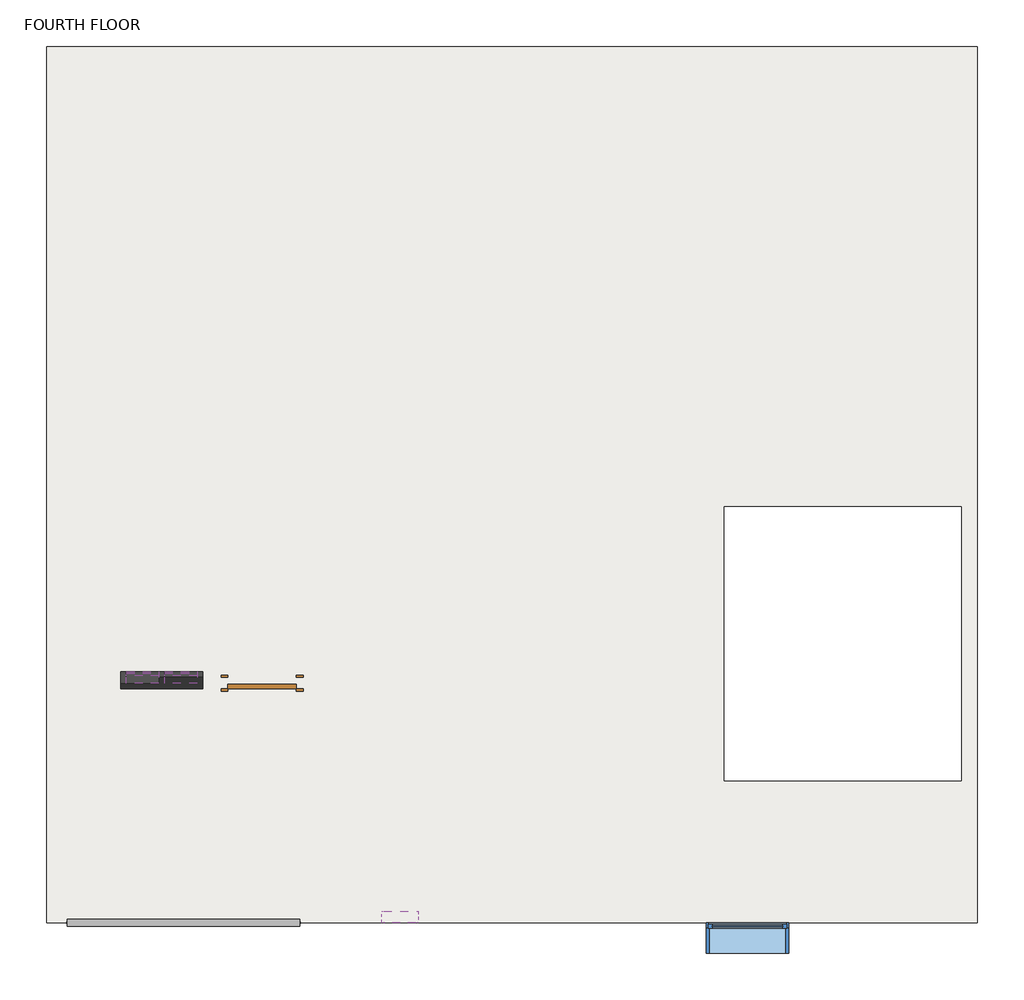
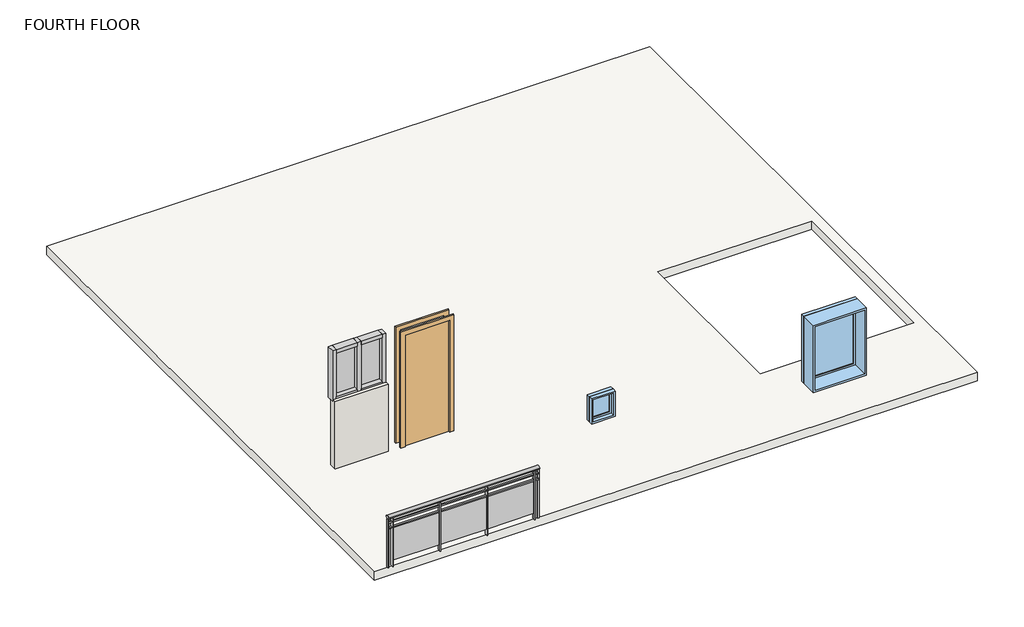
# One storey: 7 members, 2 plates, 2 windows, 1 door, 1 railing, 1 slab, 1 wall.
"""IFC4 building model written with IfcOpenShell, lengths in millimetres."""

from ifc_helpers import new_model, si_unit, point, frame, origin, place, context, project, spatial, polyline, ellipse_curve, trimmed, outline, extrude, transform, mapped, element, save
from ifc_brep_helpers import plane_surface, extruded_surface, advanced_brep
from components import door_e00f436c, member_d959a85f, member_843225dc, member_54f829b7, system_panel_glazed_8fc33089, fixed_bw_be0fa6e9, fixed_ven_0bde2124

model = new_model("IFC4")

# Units and contexts
model_context = context("Model", 3, world=origin())
ifc_project = project(units=[si_unit("LENGTHUNIT", "METRE", prefix="MILLI")], contexts=[model_context])

# Site, building, storey
site = spatial("IfcSite", under=ifc_project)
building = spatial("IfcBuilding", under=site)
storey = spatial("IfcBuildingStorey", under=building, Name="FOURTH FLOOR", Elevation=12192.0)

# Door
placement = place(None, origin())
door_shape = door_e00f436c(model_context)
element("IfcDoor", 1, ObjectType="Single-Flush : 36\" x 84\"", at=placement, inside=storey, context=model_context, shape_type="MappedRepresentation", body=[
    mapped(door_shape, transform((-4124.5569651, 3118.5055142, 12192.0), x_axis=(1.0, 0.0, 0.0), y_axis=(0.0, 1.0, 0.0), z_axis=(0.0, 0.0, 1.0))),
])

# Members
member_shape = member_d959a85f(model_context)
element("IfcMember", 2, ObjectType="Rectangular Mullion : 2.5\" x 5\" rectangular", at=placement, inside=storey, context=model_context, shape_type="MappedRepresentation", body=[
    mapped(member_shape, transform((-4784.9569651, 3182.0055142, 13381.4584417), x_axis=(1.0, 0.0, 0.0), y_axis=(0.0, -1.0, 0.0), z_axis=(0.0, 0.0, -1.0))),
])
element("IfcMember", 3, ObjectType="Rectangular Mullion : 2.5\" x 5\" rectangular", at=placement, inside=storey, context=model_context, shape_type="MappedRepresentation", body=[
    mapped(member_shape, transform((-5699.3569651, 3182.0055142, 14300.2), x_axis=(-1.0, 0.0, 0.0), y_axis=(0.0, -1.0, 0.0), z_axis=(0.0, 0.0, 1.0))),
])
member_2_shape = member_843225dc(model_context)
element("IfcMember", 4, ObjectType="Rectangular Mullion : 2.5\" x 5\" rectangular", at=placement, inside=storey, context=model_context, shape_type="MappedRepresentation", body=[
    mapped(member_2_shape, transform((-4848.4569651, 3182.0055142, 14300.2), x_axis=(0.0, 0.0, 1.0), y_axis=(0.0, -1.0, 0.0), z_axis=(1.0, 0.0, 0.0))),
])
element("IfcMember", 5, ObjectType="Rectangular Mullion : 2.5\" x 5\" rectangular", at=placement, inside=storey, context=model_context, shape_type="MappedRepresentation", body=[
    mapped(member_2_shape, transform((-5273.9069651, 3182.0055142, 14300.2), x_axis=(0.0, 0.0, 1.0), y_axis=(0.0, -1.0, 0.0), z_axis=(1.0, 0.0, 0.0))),
])
element("IfcMember", 6, ObjectType="Rectangular Mullion : 2.5\" x 5\" rectangular", at=placement, inside=storey, context=model_context, shape_type="MappedRepresentation", body=[
    mapped(member_2_shape, transform((-5635.8569651, 3182.0055142, 13381.4584417), x_axis=(0.0, 0.0, -1.0), y_axis=(0.0, -1.0, 0.0), z_axis=(-1.0, 0.0, 0.0))),
])
element("IfcMember", 7, ObjectType="Rectangular Mullion : 2.5\" x 5\" rectangular", at=placement, inside=storey, context=model_context, shape_type="MappedRepresentation", body=[
    mapped(member_2_shape, transform((-5210.4069651, 3182.0055142, 13381.4584417), x_axis=(0.0, 0.0, -1.0), y_axis=(0.0, -1.0, 0.0), z_axis=(-1.0, 0.0, 0.0))),
])
member_3_shape = member_54f829b7(model_context)
element("IfcMember", 8, ObjectType="Rectangular Mullion : 2.5\" x 5\" rectangular", at=placement, inside=storey, context=model_context, shape_type="MappedRepresentation", body=[
    mapped(member_3_shape, transform((-5242.1569651, 3182.0055142, 13381.4584417), x_axis=(1.0, 0.0, 0.0), y_axis=(0.0, -1.0, 0.0), z_axis=(0.0, 0.0, -1.0))),
])

# Plates
system_panel_glazed_shape = system_panel_glazed_8fc33089(model_context)
element("IfcPlate", 9, ObjectType="System Panel : Glazed", at=placement, inside=storey, context=model_context, shape_type="MappedRepresentation", body=[
    mapped(system_panel_glazed_shape, transform((-5454.8819651, 3182.0055142, 13444.9584417), x_axis=(1.0, 0.0, 0.0), y_axis=(0.0, 1.0, 0.0), z_axis=(0.0, 0.0, 1.0))),
])
element("IfcPlate", 10, ObjectType="System Panel : Glazed", at=placement, inside=storey, context=model_context, shape_type="MappedRepresentation", body=[
    mapped(system_panel_glazed_shape, transform((-5029.4319651, 3182.0055142, 13444.9584417), x_axis=(1.0, 0.0, 0.0), y_axis=(0.0, 1.0, 0.0), z_axis=(0.0, 0.0, 1.0))),
])

# Railing
element("IfcRailing", 11, ObjectType="Glass Panel - Bottom Fill", at=placement, inside=storey, context=model_context, shape_type="SolidModel", body=[
    advanced_brep(
    [(-6296.2569651, 489.6055142, 13106.4), (-6296.2569651, 413.4055142, 13106.4), (-3705.4569651, 489.6055142, 13106.4), (-3705.4569651, 413.4055142, 13106.4)],
    [
        (0, 1, ellipse_curve(frame((-6296.2569651, 451.5055142, 13106.4), z_axis=(-1.0, 0.0, 0.0), x_axis=(0.0, -1.0, 0.0)), 38.1, 28.575)),
        (1, 0, ellipse_curve(frame((-6296.2569651, 451.5055142, 13106.4), z_axis=(-1.0, 0.0, 0.0), x_axis=(0.0, -1.0, 0.0)), 38.1, 28.575)),
        (2, 3, ellipse_curve(frame((-3705.4569651, 451.5055142, 13106.4), z_axis=(1.0, 0.0, 0.0), x_axis=(0.0, -1.0, 0.0)), 38.1, 28.575)),
        (3, 2, ellipse_curve(frame((-3705.4569651, 451.5055142, 13106.4), z_axis=(1.0, 0.0, 0.0), x_axis=(0.0, -1.0, 0.0)), 38.1, 28.575)),
        (0, 2),
        (3, 1),
    ],
    [
        plane_surface(frame((-6296.2569651, 451.5055142, 13106.4), z_axis=(-1.0, 0.0, 0.0), x_axis=(0.0, 1.0, 0.0))),
        plane_surface(frame((-3705.4569651, 451.5055142, 13106.4), z_axis=(1.0, 0.0, 0.0), x_axis=(0.0, 1.0, 0.0))),
        extruded_surface(trimmed(ellipse_curve(frame((-3705.4569651, 451.5055142, 13106.4), z_axis=(-1.0, 0.0, 0.0), x_axis=(0.0, -1.0, 0.0)), 38.1, 28.575), [point((-3705.4569651, 489.6055142, 13106.4))], [point((-3705.4569651, 413.4055142, 13106.4))], True, "CARTESIAN"), (-2590.8, 0.0, 0.0), 2590.8),
        extruded_surface(trimmed(ellipse_curve(frame((-3705.4569651, 451.5055142, 13106.4), z_axis=(-1.0, 0.0, 0.0), x_axis=(0.0, -1.0, 0.0)), 38.1, 28.575), [point((-3705.4569651, 413.4055142, 13106.4))], [point((-3705.4569651, 489.6055142, 13106.4))], True, "CARTESIAN"), (-2590.8, 0.0, 0.0), 2590.8),
    ],
    [
        (0, [[1, 2]]),
        (1, [[3, 4]]),
        (2, [[-1, 5, -4, 6]]),
        (3, [[-2, -6, -3, -5]]),
    ],
),
    extrude(outline(polyline([(-6296.2569651, 438.8055142), (-6296.2569651, 464.2055142), (-3705.4569651, 464.2055142), (-3705.4569651, 438.8055142), (-6296.2569651, 438.8055142)])), frame((0.0, 0.0, 12992.1), z_axis=(0.0, 0.0, 1.0), x_axis=(1.0, 0.0, 0.0)), (0.0, 0.0, 1.0), 25.4),
    extrude(outline(polyline([(-6296.2569651, 438.8055142), (-6296.2569651, 464.2055142), (-3705.4569651, 464.2055142), (-3705.4569651, 438.8055142), (-6296.2569651, 438.8055142)])), frame((0.0, 0.0, 12890.5), z_axis=(0.0, 0.0, 1.0), x_axis=(1.0, 0.0, 0.0)), (0.0, 0.0, 1.0), 25.4),
    extrude(outline(polyline([(-3788.0069651, 426.1055142), (-3788.0069651, 476.9055142), (-3775.3069651, 476.9055142), (-3775.3069651, 426.1055142), (-3788.0069651, 426.1055142)])), frame((0.0, 0.0, 12192.0), z_axis=(0.0, 0.0, 1.0), x_axis=(1.0, 0.0, 0.0)), (0.0, 0.0, 1.0), 885.6788223),
    extrude(outline(polyline([(-4594.4569651, 458.0406712), (-3781.6569651, 458.0406712), (-3781.6569651, 451.6906712), (-4594.4569651, 451.6906712), (-4594.4569651, 458.0406712)])), frame((0.0, 0.0, 12293.6), z_axis=(0.0, 0.0, 1.0), x_axis=(1.0, 0.0, 0.0)), (0.0, 0.0, 1.0), 596.9),
    extrude(outline(polyline([(-4600.8069651, 426.1055142), (-4600.8069651, 476.9055142), (-4588.1069651, 476.9055142), (-4588.1069651, 426.1055142), (-4600.8069651, 426.1055142)])), frame((0.0, 0.0, 12192.0), z_axis=(0.0, 0.0, 1.0), x_axis=(1.0, 0.0, 0.0)), (0.0, 0.0, 1.0), 885.6788223),
    extrude(outline(polyline([(-5407.2569651, 458.0406712), (-4594.4569651, 458.0406712), (-4594.4569651, 451.6906712), (-5407.2569651, 451.6906712), (-5407.2569651, 458.0406712)])), frame((0.0, 0.0, 12293.6), z_axis=(0.0, 0.0, 1.0), x_axis=(1.0, 0.0, 0.0)), (0.0, 0.0, 1.0), 596.9),
    extrude(outline(polyline([(-5413.6069651, 426.1055142), (-5413.6069651, 476.9055142), (-5400.9069651, 476.9055142), (-5400.9069651, 426.1055142), (-5413.6069651, 426.1055142)])), frame((0.0, 0.0, 12192.0), z_axis=(0.0, 0.0, 1.0), x_axis=(1.0, 0.0, 0.0)), (0.0, 0.0, 1.0), 885.6788223),
    extrude(outline(polyline([(-6220.0569651, 458.0406712), (-5407.2569651, 458.0406712), (-5407.2569651, 451.6906712), (-6220.0569651, 451.6906712), (-6220.0569651, 458.0406712)])), frame((0.0, 0.0, 12293.6), z_axis=(0.0, 0.0, 1.0), x_axis=(1.0, 0.0, 0.0)), (0.0, 0.0, 1.0), 596.9),
    extrude(outline(polyline([(-6226.4069651, 426.1055142), (-6226.4069651, 476.9055142), (-6213.7069651, 476.9055142), (-6213.7069651, 426.1055142), (-6226.4069651, 426.1055142)])), frame((0.0, 0.0, 12192.0), z_axis=(0.0, 0.0, 1.0), x_axis=(1.0, 0.0, 0.0)), (0.0, 0.0, 1.0), 885.6788223),
    extrude(outline(polyline([(-3718.1569651, 441.9805142), (-3718.1569651, 461.0305142), (-3699.1069651, 461.0305142), (-3699.1069651, 441.9805142), (-3718.1569651, 441.9805142)])), frame((0.0, 0.0, 12192.0), z_axis=(0.0, 0.0, 1.0), x_axis=(1.0, 0.0, 0.0)), (0.0, 0.0, 1.0), 885.6788223),
    extrude(outline(polyline([(-6302.6069651, 441.9805142), (-6302.6069651, 461.0305142), (-6283.5569651, 461.0305142), (-6283.5569651, 441.9805142), (-6302.6069651, 441.9805142)])), frame((0.0, 0.0, 12192.0), z_axis=(0.0, 0.0, 1.0), x_axis=(1.0, 0.0, 0.0)), (0.0, 0.0, 1.0), 885.6788223),
])

# Slab
element("IfcSlab", 12, ObjectType="Generic - 12\"", at=placement, inside=storey, context=model_context, shape_type="SweptSolid", body=[
    extrude(outline(polyline([(3838.3430349, 10205.1055142), (3838.3430349, 451.5055142), (-6524.8569651, 451.5055142), (-6524.8569651, 10205.1055142), (3838.3430349, 10205.1055142)]), holes=[polyline([(3660.5430349, 5080.6555142), (1018.9430349, 5080.6555142), (1018.9430349, 2032.6555142), (3660.5430349, 2032.6555142), (3660.5430349, 5080.6555142)])]), frame((0.0, 0.0, 12039.6), z_axis=(0.0, 0.0, 1.0), x_axis=(1.0, 0.0, 0.0)), (0.0, 0.0, 1.0), 152.4),
])

# Wall
element("IfcWall", 13, ObjectType="5\"", at=placement, inside=storey, context=model_context, shape_type="SweptSolid", body=[
    extrude(outline(polyline([(-4784.9569651, 3055.0055142), (-5699.3569651, 3055.0055142), (-5699.3569651, 3182.0055142), (-4784.9569651, 3182.0055142), (-4784.9569651, 3055.0055142)])), frame((0.0, 0.0, 11252.2), z_axis=(0.0, 0.0, 1.0), x_axis=(1.0, 0.0, 0.0)), (0.0, 0.0, 1.0), 2159.0),
])

# Windows
fixed_bw_shape = fixed_bw_be0fa6e9(model_context)
element("IfcWindow", 14, ObjectType="Fixed : BW", at=placement, inside=storey, context=model_context, shape_type="MappedRepresentation", body=[
    mapped(fixed_bw_shape, transform((1316.0073388, 281.3921573, 12166.6), x_axis=(1.0, 0.0, 0.0), y_axis=(0.0, 1.0, 0.0), z_axis=(0.0, 0.0, 1.0))),
])
fixed_ven_shape = fixed_ven_0bde2124(model_context)
element("IfcWindow", 15, ObjectType="Fixed : VEN", at=placement, inside=storey, context=model_context, shape_type="MappedRepresentation", body=[
    mapped(fixed_ven_shape, transform((-2549.7569651, 515.0055142, 12656.695937), x_axis=(1.0, 0.0, 0.0), y_axis=(0.0, 1.0, 0.0), z_axis=(0.0, 0.0, 1.0))),
])

save(model, "model.ifc")

# Revit data of these elements
# Type "Single-Flush : 36\" x 84\""
#   Type Mark = "1"
#   Construction Type Id = "MDOOR"
#   Assembly Code = "C1020"
#   Analytic Construction = "Metal"
#   Thickness = 0' - 2"
#   Heat Transfer Coefficient (U) = 0.651978 BTU/(h·ft²·°F)
#   Height = 6' - 8"
#   Trim Projection Ext = 0' - 1"
#   Trim Projection Int = 0' - 1"
#   Trim Width = 0' - 3"
#   Width = 2' - 6"
#   Define Thermal Properties by = 1
#   Define Thermal Properties by = 1
#   Door Material = Door - Panel
#   Frame Material = Door - Frame
#   Visual Light Transmittance = 0
#   Solar Heat Gain Coefficient = 0
#   Function = (empty or 0)
#   Wall Closure = (empty or 0)
# Type "Rectangular Mullion : 2.5\" x 5\" rectangular"
#   built-in parameter 1007304 = 0.416667 (stored number, unit not read)
#   built-in parameter 1007301 = 0.104167 (stored number, unit not read)
#   built-in parameter 1007300 = 0.104167 (stored number, unit not read)
# Type "System Panel : Glazed"
#   Construction Type Id = "GSP4R"
#   Analytic Construction = "1/8 in Pilkington single glazing"
#   Visual Light Transmittance = 0.9
#   Solar Heat Gain Coefficient = 0.86
#   Heat Transfer Coefficient (U) = 1.18115 BTU/(h·ft²·°F)
#   Define Thermal Properties by = 1
# Type "Glass Panel - Bottom Fill"
#   Assembly Code = "C2010400"
#   built-in parameter 1008612 = 0.0416667 (stored number, unit not read)
#   built-in parameter 1008611 = 0.0416667 (stored number, unit not read)
#   built-in parameter 1008609 = 0.333333 (stored number, unit not read)
#   built-in parameter 1008604 = 0.166667 (stored number, unit not read)
#   built-in parameter 1008603 = 0.166667 (stored number, unit not read)
#   Railing Height = 3' - 0"
#   built-in parameter 1008630 = 2
#   built-in parameter 1008610 = 2
#   built-in parameter 1008618 = Baluster - Square : 3/4"
# Type "Generic - 12\""
#   Assembly Code = "B1010"
#   Function = 0
#   Layers, outside or top first: 0' - 6" no material (function 1)
# Type "5\""
#   Assembly Code = "B2010"
#   Layers, outside or top first: 0' - 5" "Concrete Masonry Units" (function 1)
# Type "Fixed : BW"
#   Type Mark = "18"
#   Construction Type Id = "GSP4R"
#   Assembly Code = "B2020100"
#   Analytic Construction = "1/8 in Pilkington single glazing"
#   Visual Light Transmittance = 0.9
#   Solar Heat Gain Coefficient = 0.78
#   Heat Transfer Coefficient (U) = 0.6496 BTU/(h·ft²·°F)
#   Height = 4' - 0"
#   Default Sill Height = 3' - 0"
#   Width = 3' - 0"
#   Window Inset = 0' - 0 3/4"
#   Define Thermal Properties by = 1
#   Glass Pane Material = Glass
#   Sash Material = Sash
#   Wall Closure = (empty or 0)
# Type "Fixed : VEN"
#   Type Mark = "19"
#   Construction Type Id = "GSP4R"
#   Assembly Code = "B2020100"
#   Analytic Construction = "1/8 in Pilkington single glazing"
#   Visual Light Transmittance = 0.9
#   Solar Heat Gain Coefficient = 0.78
#   Heat Transfer Coefficient (U) = 0.6496 BTU/(h·ft²·°F)
#   Height = 1' - 6"
#   Default Sill Height = 3' - 0"
#   Width = 1' - 4"
#   Window Inset = 0' - 0 3/4"
#   Define Thermal Properties by = 1
#   Glass Pane Material = Glass
#   Sash Material = Sash
#   Wall Closure = (empty or 0)
# Element 1 (IfcDoor, "Single-Flush : 36\" x 84\"")
#   Phase Created = New Construction
#   Materials on its faces: "Door - Frame", "Door - Panel"
# Elements 2, 3, 4, 5, 6, 7, 8 (IfcMember, "Rectangular Mullion : 2.5\" x 5\" rectangular")
#   Phase Created = New Construction
#   Materials on its faces: "Aluminum"
# Elements 9, 10 (IfcPlate, "System Panel : Glazed")
#   Phase Created = New Construction
#   Materials on its faces: "Glass"
# Element 11 (IfcRailing, "Glass Panel - Bottom Fill")
#   Phase Created = New Construction
#   Materials on its faces: "Glass"
# Element 12 (IfcSlab, "Generic - 12\"")
#   Height Offset From Level = 0' - 0"
#   Phase Created = New Construction
#   Materials on its faces: "Default Floor", "1 wall brown"
# Element 13 (IfcWall, "5\"")
#   built-in parameter 1001111 = -3' - 1"
#   Top Offset = 0' - 0"
#   Base Offset = -3' - 1"
#   Unconnected Height = 7' - 1"
#   wall height = 7' - 1"
#   Phase Created = New Construction
#   Base Constraint = FOURTH FLOOR
#   Materials on its faces: "Concrete Masonry Units", "1 wall white"
# Element 14 (IfcWindow, "Fixed : BW")
#   Mark = "7"
#   Phase Created = New Construction
#   Materials on its faces: "Sash", "Glass"
# Element 15 (IfcWindow, "Fixed : VEN")
#   Mark = "13"
#   Phase Created = New Construction
#   Materials on its faces: "Sash", "Glass"
# Materials
#   "Door - Panel": class "Wood", colour RGB 210 159 95, transparency 0, Cost = 0
#   "Door - Frame": colour RGB 118 70 51, transparency 0, Cost = 0
#   "Concrete Masonry Units": class "Masonry", colour RGB 227 227 227, transparency 0, Description = "Concrete masonry units", Cost = 0
#   "Glass": class "Glass", colour RGB 0 128 192, transparency 0.75, Description = "Soda Lime Glass", Cost = 0
#   "Sash": class "Wood", colour RGB 224 178 126, transparency 0, Cost = 0
#   "Aluminum": class "Metal", colour RGB 247 247 247, transparency 0, Description = "Aluminum 6061", Cost = 0
#   "Default Floor": colour RGB 128 128 128, transparency 0, Cost = 0
#   "1 wall brown": class "Generic", colour RGB 61 46 37, transparency 0, Cost = 0
#   "1 wall white": class "Generic", colour RGB 244 245 241, transparency 0, Cost = 0
